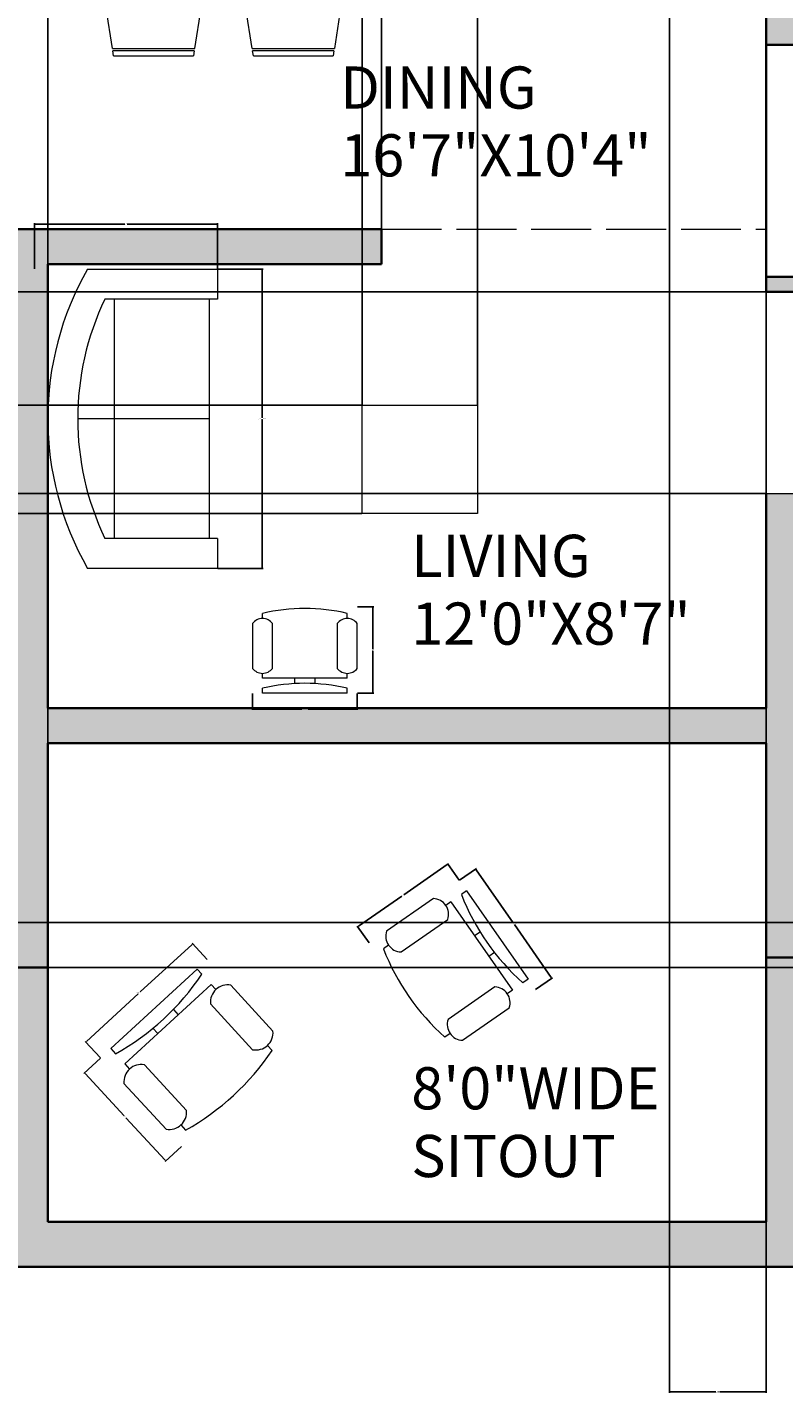
# Model space of a CAD drawing. Units: inches. Extents: x -12 to 539, y -477 to 51.
# Tile 3 of 6: x 173 to 325, y -477 to -203. Entities that reach past the tile are written whole.
import ezdxf

# ---------------------------------------------------------------- set-up
doc = ezdxf.new("R2010")
doc.units = ezdxf.units.IN
doc.header["$MEASUREMENT"] = 0
doc.linetypes.add('ACAD_ISO02W100', pattern=[15, 12, -3])
for name, color, linetype, lineweight in [('A-ANNO-DIMS', 2, 'Continuous', 18), ('A-AREA-IDEN', 7, 'Continuous', 18), ('A-FLOR-CASE', 9, 'Continuous', 18), ('A-FURN', 8, 'Continuous', 18), ('A-WALL', 7, 'Continuous', 35), ('A-WALL-OVHD', 7, 'ACAD_ISO02W100', 18)]:
    doc.layers.add(name, color=color, linetype=linetype, lineweight=lineweight)
doc.layers.add('A-WALL-PATT', color=252, linetype='Continuous', lineweight=13, true_color=0x939598)
doc.styles.get("Standard").update_dxf_attribs({"font": 'arial.ttf'})
doc.dimstyles.get("Standard").update_dxf_attribs({"dimtxt": 0.18, "dimasz": 0.18, "dimexe": 0.18, "dimexo": 0.0625, "dimgap": 0.09, "dimtad": 0, "dimtih": 1, "dimtoh": 1, "dimdec": 0, "dimzin": 0, "dimdsep": 46, "dimlunit": 3, "dimtxsty": 'Standard', "dimcen": 0.09, "dimadec": 0, "dimazin": 0, "dimtfac": 1, "dimtdec": 0, "dimtofl": 0, "dimtmove": 0, "dimatfit": 3, "dimfxl": 1, "dimtolj": 1, "dimtzin": 0, "dimarcsym": 0})

# ---------------------------------------------------------------- blocks, each defined once
blk = doc.blocks.new('Dining Set - 36 x 72 in.')
for p, q in [((-22, 27.5), (-22.1562, 26.50042)), ((-22, 27.5), (-6, 27.5)), ((-5.8437, 26.49966), (-6, 27.5)), ((6, 27.5), (5.8438, 26.50042)), ((6, 27.5), (22, 27.5)), ((22.1563, 26.49966), (22, 27.5)), ((-22.2343, 26.00059), (-23.4847, 17.99762)), ((-22.2304, 26), (-5.7608, 26)), ((-5.8416, 26.5), (-22.1534, 26.5)), ((-4.5152, 17.99762), (-5.7655, 25.99926)), ((5.7657, 26.00059), (4.5153, 17.99762)), ((5.7696, 26), (22.2392, 26)), ((22.1584, 26.5), (5.8466, 26.5)), ((23.4848, 17.99762), (22.2345, 25.99926)), ((36, 18), (-36, 18)), ((-36, 18), (-36, -18)), ((36, -18), (36, 18)), ((-44.0006, 8.23428), (-35.9976, 9.48474)), ((-44, 8.23041), (-44, -8.23915)), ((44.0006, 8.23428), (35.9976, 9.48474)), ((44, 8.23041), (44, -8.23915)), ((-45.5, 8), (-44.5004, 8.15617)), ((-45.5, 8), (-45.5, -8)), ((-44.5, -8.15843), (-44.5, 8.15338)), ((44.5, -8.15843), (44.5, 8.15338)), ((45.5, 8), (44.5005, 8.15617)), ((45.5, 8), (45.5, -8)), ((-44.4997, -8.15631), (-45.5, -8)), ((44.4997, -8.15631), (45.5, -8)), ((-35.9976, -9.48476), (-43.9993, -8.2345)), ((35.9976, -9.48476), (43.9993, -8.2345)), ((-36, -18), (36, -18)), ((-22.2343, -26.0006), (-23.4847, -17.99762)), ((-4.5152, -17.99762), (-5.7655, -25.99928)), ((5.7657, -26.0006), (4.5153, -17.99762)), ((23.4848, -17.99762), (22.2345, -25.99928)), ((-22.2304, -26), (-5.7608, -26)), ((-22, -27.5), (-22.1562, -26.50044)), ((-5.8416, -26.5), (-22.1534, -26.5)), ((-5.8437, -26.49967), (-6, -27.5)), ((5.7696, -26), (22.2392, -26)), ((6, -27.5), (5.8438, -26.50044)), ((22.1584, -26.5), (5.8466, -26.5)), ((22.1563, -26.49967), (22, -27.5)), ((-22, -27.5), (-6, -27.5)), ((6, -27.5), (22, -27.5))]:
    blk.add_line(p, q)
for points in [[(-36, 15), (-31.1772, 14.97754), (-26.8079, 14.91406), (-22.8538, 14.81543), (-19.276, 14.6875), (-16.0362, 14.53613), (-13.0957, 14.36718), (-10.4159, 14.18652), (-7.9583, 14), (-5.6904, 13.81315), (-3.6035, 13.63021), (-1.6954, 13.45508), (0.0365, 13.29166), (1.5945, 13.14388), (2.9811, 13.01562), (4.1988, 12.9108), (5.25, 12.83333), (6.1393, 12.78613), (6.8802, 12.76823), (7.4883, 12.77767), (7.9792, 12.8125), (8.3685, 12.87077), (8.6719, 12.95052), (8.9049, 13.0498), (9.0833, 13.16666), (9.2205, 13.29899), (9.3216, 13.44401), (9.3895, 13.59879), (9.4271, 13.76041), (9.4373, 13.92594), (9.4232, 14.09245), (9.3875, 14.257), (9.3333, 14.41666), (9.2638, 14.56917), (9.1836, 14.71484), (9.0975, 14.85465), (9.0104, 14.98958), (8.9272, 15.1206), (8.8529, 15.2487), (8.7922, 15.37483), (8.75, 15.5), (8.7305, 15.62467), (8.7344, 15.74739), (8.7617, 15.86621), (8.8125, 15.97916), (8.8867, 16.08431), (8.9844, 16.17968), (9.1055, 16.26334), (9.25, 16.33333), (9.4189, 16.38802), (9.6172, 16.42708), (9.8506, 16.45052), (10.125, 16.45833), (10.4463, 16.45052), (10.8203, 16.42708), (11.2529, 16.38802), (11.75, 16.33333), (12.3184, 16.26318), (12.9694, 16.17838), (13.7151, 16.07991), (14.5677, 15.96875), (15.5395, 15.84586), (16.6426, 15.71224), (17.8893, 15.56884), (19.2917, 15.41666), (20.859, 15.25667), (22.5879, 15.08984), (24.4721, 14.91715), (26.5052, 14.73958), (28.6809, 14.5581), (30.9929, 14.3737), (33.4347, 14.18733), (36, 14)], [(-36, 10), (-28.9766, 10.14274), (-23.1725, 10.20442), (-18.4241, 10.19775), (-14.5677, 10.13541), (-11.4399, 10.03011), (-8.877, 9.89453), (-6.7154, 9.74137), (-4.7917, 9.58333), (-2.9698, 9.43082), (-1.2246, 9.28515), (0.4415, 9.14534), (2.026, 9.01041), (3.5266, 8.87939), (4.9408, 8.7513), (6.266, 8.62516), (7.5, 8.5), (8.6411, 8.37549), (9.6914, 8.2539), (10.6538, 8.13818), (11.5312, 8.03125), (12.3267, 7.93603), (13.043, 7.85547), (13.6831, 7.79248), (14.25, 7.75), (14.7471, 7.7303), (15.1797, 7.73307), (15.5537, 7.75732), (15.875, 7.80208), (16.1494, 7.86637), (16.3828, 7.94922), (16.5811, 8.04964), (16.75, 8.16666), (16.8944, 8.29915), (17.0143, 8.44531), (17.1089, 8.60319), (17.1771, 8.77083), (17.218, 8.94629), (17.2305, 9.1276), (17.2137, 9.31282), (17.1667, 9.5), (17.0895, 9.6875), (16.987, 9.875), (16.8649, 10.0625), (16.7292, 10.25), (16.5856, 10.4375), (16.4401, 10.625), (16.2985, 10.8125), (16.1667, 11), (16.05, 11.18733), (15.9518, 11.3737), (15.8752, 11.5581), (15.8229, 11.73958), (15.798, 11.91715), (15.8034, 12.08984), (15.842, 12.25667), (15.9167, 12.41666), (16.0295, 12.56836), (16.1784, 12.70833), (16.3605, 12.83268), (16.5729, 12.9375), (16.8127, 13.01888), (17.0768, 13.07291), (17.3625, 13.0957), (17.6667, 13.08333), (17.9894, 13.03312), (18.3418, 12.94726), (18.7382, 12.82918), (19.1927, 12.68229), (19.7195, 12.51001), (20.3327, 12.31575), (21.0465, 12.10294), (21.875, 11.875), (22.8357, 11.63354), (23.959, 11.37304), (25.2786, 11.08618), (26.8282, 10.76562), (28.6414, 10.40405), (30.752, 9.99414), (33.1936, 9.52856), (36, 9)], [(-36, 5.5), (-30.7157, 5.3348), (-26.069, 5.20963), (-21.9946, 5.11767), (-18.4271, 5.05208), (-15.3009, 5.00602), (-12.5508, 4.97265), (-10.1112, 4.94515), (-7.9167, 4.91666), (-5.909, 4.88167), (-4.0586, 4.83984), (-2.3429, 4.79215), (-0.7396, 4.73958), (0.7739, 4.6831), (2.22, 4.6237), (3.6213, 4.56233), (5, 4.5), (6.373, 4.43782), (7.7344, 4.3776), (9.0723, 4.32129), (10.375, 4.27083), (11.6309, 4.22819), (12.8281, 4.19531), (13.9551, 4.17415), (15, 4.16666), (15.954, 4.17448), (16.819, 4.19791), (17.6001, 4.23698), (18.3021, 4.29166), (18.9299, 4.36198), (19.4883, 4.44791), (19.9823, 4.54948), (20.4167, 4.66666), (20.7969, 4.79899), (21.1302, 4.94401), (21.4245, 5.09879), (21.6875, 5.26041), (21.9271, 5.42594), (22.1511, 5.59245), (22.3672, 5.757), (22.5834, 5.91666), (22.8065, 6.06868), (23.0404, 6.21093), (23.2879, 6.34147), (23.5521, 6.45833), (23.8358, 6.55957), (24.142, 6.64323), (24.4735, 6.70735), (24.8334, 6.75), (25.2235, 6.76969), (25.642, 6.76692), (26.0858, 6.74267), (26.5521, 6.69791), (27.0379, 6.63362), (27.5404, 6.55078), (28.0565, 6.45036), (28.5834, 6.33333), (29.1242, 6.19987), (29.7071, 6.04687), (30.3661, 5.87044), (31.1354, 5.66666), (32.0493, 5.43164), (33.142, 5.16146), (34.4475, 4.85221), (36, 4.5)], [(-36, -1), (-30.7915, -0.6591), (-26.0195, -0.38216), (-21.6519, -0.16284), (-17.6563, 0.00521), (-14.0005, 0.12833), (-10.6523, 0.21289), (-7.5796, 0.26522), (-4.75, 0.29166), (-2.134, 0.29793), (0.2878, 0.28711), (2.5317, 0.26163), (4.6146, 0.22396), (6.5529, 0.17651), (8.3633, 0.12174), (10.0623, 0.06209), (11.6667, 0), (13.1899, -0.06201), (14.6341, -0.1211), (15.9982, -0.17432), (17.2813, -0.21875), (18.4823, -0.25147), (19.6003, -0.26953), (20.6343, -0.27002), (21.5834, -0.25), (22.4481, -0.20768), (23.2357, -0.14584), (23.9549, -0.06836), (24.6146, 0.02083), (25.2235, 0.11784), (25.7904, 0.21875), (26.3241, 0.31966), (26.8334, 0.41666), (27.3265, 0.50618), (27.8099, 0.58593), (28.2894, 0.65397), (28.7709, 0.70833), (29.2601, 0.74707), (29.763, 0.76823), (30.2855, 0.76985), (30.8334, 0.75), (31.4088, 0.70784), (31.9994, 0.64713), (32.589, 0.57275), (33.1615, 0.48958), (33.7008, 0.4025), (34.1908, 0.3164), (34.6153, 0.23616), (34.9584, 0.16666), (35.2099, 0.11165), (35.3848, 0.07031), (35.504, 0.04069), (35.5886, 0.02083), (35.6594, 0.00879), (35.7377, 0.0026), (35.8442, 0.00032), (36, 0)], [(-36, -6.5), (-27.1843, -6.31267), (-20.084, -6.1263), (-14.469, -5.9419), (-10.1094, -5.76042), (-6.7752, -5.58285), (-4.2363, -5.41016), (-2.2629, -5.24333), (-0.625, -5.08334), (0.8708, -4.93099), (2.2715, -4.78646), (3.5872, -4.64974), (4.8281, -4.52084), (6.0046, -4.39974), (7.127, -4.28646), (8.2053, -4.18099), (9.25, -4.08334), (10.2705, -3.99382), (11.2734, -3.91407), (12.2647, -3.84603), (13.25, -3.79167), (14.2354, -3.75293), (15.2266, -3.73177), (16.2295, -3.73015), (17.25, -3.75), (18.2912, -3.79248), (19.3451, -3.85547), (20.4009, -3.93604), (21.4479, -4.03125), (22.4754, -4.13819), (23.4727, -4.25391), (24.4289, -4.37549), (25.3334, -4.5), (26.1785, -4.62492), (26.9694, -4.74935), (27.7145, -4.87281), (28.4219, -4.99479), (29.1, -5.11483), (29.7572, -5.23242), (30.4016, -5.34709), (31.0417, -5.45834), (31.6837, -5.56437), (32.3262, -5.65821), (32.9658, -5.73153), (33.599, -5.77604), (34.2224, -5.78345), (34.8327, -5.74545), (35.4264, -5.65373), (36, -5.5)], [(-36, -10), (-26.4022, -9.81299), (-18.4675, -9.62891), (-11.9839, -9.45069), (-6.7396, -9.28125), (-2.5226, -9.12354), (0.8789, -8.98047), (3.6769, -8.85498), (6.0833, -8.75), (8.2767, -8.66765), (10.3021, -8.60677), (12.1712, -8.56543), (13.8958, -8.54167), (15.4876, -8.53353), (16.9583, -8.53907), (18.3197, -8.55632), (19.5834, -8.58334), (20.7616, -8.61841), (21.8685, -8.66081), (22.9188, -8.71004), (23.9271, -8.76563), (24.9081, -8.82707), (25.8763, -8.89388), (26.8465, -8.96558), (27.8334, -9.04167), (28.8474, -9.12118), (29.8828, -9.20117), (30.93, -9.27824), (31.9792, -9.34896), (33.0205, -9.40991), (34.0443, -9.45768), (35.0407, -9.48885), (36, -9.5)], [(-36, -14.5), (-30.0881, -14.33513), (-25.0332, -14.21224), (-20.7312, -14.12647), (-17.0781, -14.07292), (-13.97, -14.04671), (-11.3027, -14.04297), (-8.9724, -14.05681), (-6.875, -14.08334), (-4.9224, -14.11833), (-3.0905, -14.16016), (-1.3709, -14.20785), (0.2448, -14.26042), (1.7647, -14.3169), (3.1973, -14.3763), (4.5507, -14.43767), (5.8333, -14.5), (7.0554, -14.5621), (8.235, -14.62175), (9.3922, -14.67652), (10.5469, -14.72396), (11.7192, -14.76164), (12.929, -14.78711), (14.1965, -14.79794), (15.5417, -14.79167), (16.9933, -14.76424), (18.6152, -14.70508), (20.4804, -14.60197), (22.6615, -14.44271), (25.2312, -14.21509), (28.2624, -13.9069), (31.8277, -13.50594), (36, -13)]]:
    blk.add_lwpolyline(points)
blk = doc.blocks.new('Sofa - Roundback Loveseat 5 ft.')
for p, q in [((0, -32.44198), (0, -5.99998)), ((-24, -33.99998), (-24, -11.46958)), ((-23.9998, -13.38178), (23.99986, -13.38178)), ((24.00004, -33.99998), (24.00004, -11.46958)), ((-24, -32.44198), (24.00004, -32.44198))]:
    blk.add_line(p, q)
for points in [[(-24, -33.99998), (-30, -33.99998), (-30, -7.99998)], [(30.00004, -7.99998), (30.00004, -33.99998), (24.00004, -33.99998)]]:
    blk.add_lwpolyline(points)
for centre, radius, start, end in [((0, -60.24998), 60.24998, 60.13715, 119.8628), ((0, -61.38438), 55.38444, 64.32083, 115.6792)]:
    blk.add_arc(centre, radius, start, end)
blk = doc.blocks.new('Chair - Desk')
for p, q in [((-8.5, 0), (-8.5, -1)), ((-8.5, 0), (8.5, 0)), ((8.5, 0), (8.5, -1)), ((-2, -3), (-2, -1.9355)), ((2, -1.9576), (2, -3)), ((-8.5, -3), (-8.5, -4)), ((-8.5, -3), (8.5, -3)), ((8.5, -3), (8.5, -4)), ((-10.5, -5), (-10.5, -14)), ((-6.5, -14), (-6.5, -5)), ((6.5, -5), (6.5, -14)), ((10.5, -14), (10.5, -5)), ((-8.5, -15), (-8.5, -16)), ((8.5, -15), (8.5, -16))]:
    blk.add_line(p, q)
for centre, radius, start, end in [((0, 34.625), 36.625, 256.5803, 283.4197), ((-8.5, -6.5), 2.5, 36.8699, 143.1301), ((8.5, -6.5), 2.5, 36.8699, 143.1301), ((-8.5, -12.5), 2.5, 216.8699, 323.1301), ((8.5, -12.5), 2.5, 216.8699, 323.1301), ((0, 19.625), 36.625, 256.5803, 283.4197)]:
    blk.add_arc(centre, radius, start, end)
blk = doc.blocks.new('*D13')
at = {"layer": 'A-ANNO-DIMS', "color": 0, "lineweight": -2, "transparency": 16777216}
for p, q in [((218.14, -337.07), (218.14, -340.34)), ((239.14, -337.07), (239.14, -340.34)), ((218.32, -340.16), (228.02, -340.16)), ((238.96, -340.16), (229.27, -340.16))]:
    blk.add_line(p, q, dxfattribs=at)
at = {"layer": 'A-ANNO-DIMS', "color": 0, "transparency": 16777216}
for points in [[(218.32, -340.13), (218.32, -340.19), (218.14, -340.16)], [(238.96, -340.13), (238.96, -340.19), (239.14, -340.16)]]:
    blk.add_solid(points, dxfattribs=at)
at = {"layer": 'Defpoints', "color": 0, "transparency": 16777216}
for p in [(218.14, -337.01), (239.14, -337.01), (218.14, -340.16)]:
    blk.add_point(p, dxfattribs=at)
at = {"layer": 'A-ANNO-DIMS', "color": 0, "transparency": 16777216, "insert": (228.64, -340.16), "char_height": 0.18, "attachment_point": 5}
blk.add_mtext('\\A1;CHAIR 21', dxfattribs=at)
blk = doc.blocks.new('*D14')
at = {"layer": 'A-ANNO-DIMS', "color": 0, "lineweight": -2, "transparency": 16777216}
for p, q in [((239.21, -319.67), (242.47, -319.67)), ((242.29, -319.85), (242.29, -328.16)), ((242.29, -336.83), (242.29, -328.52)), ((239.21, -337.01), (242.47, -337.01))]:
    blk.add_line(p, q, dxfattribs=at)
at = {"layer": 'A-ANNO-DIMS', "color": 0, "transparency": 16777216}
for points in [[(242.26, -319.85), (242.32, -319.85), (242.29, -319.67)], [(242.26, -336.83), (242.32, -336.83), (242.29, -337.01)]]:
    blk.add_solid(points, dxfattribs=at)
at = {"layer": 'Defpoints', "color": 0, "transparency": 16777216}
for p in [(239.14, -319.67), (239.14, -337.01), (242.29, -337.01)]:
    blk.add_point(p, dxfattribs=at)
at = {"layer": 'A-ANNO-DIMS', "color": 0, "transparency": 16777216, "insert": (242.29, -328.34), "char_height": 0.18, "attachment_point": 5}
blk.add_mtext('\\A1;17', dxfattribs=at)
blk = doc.blocks.new('*D15')
at = {"layer": 'A-ANNO-DIMS', "color": 0, "lineweight": -2, "transparency": 16777216}
for p, q in [((206.03, -387.34), (195.65, -396.89)), ((209.07, -390.39), (206.04, -387.09)), ((184.87, -406.8), (195.25, -397.25)), ((187.65, -410.08), (184.62, -406.79))]:
    blk.add_line(p, q, dxfattribs=at)
at = {"layer": 'A-ANNO-DIMS', "color": 0, "transparency": 16777216}
for points in [[(206.01, -387.32), (206.05, -387.37), (206.16, -387.22)], [(184.85, -406.77), (184.9, -406.82), (184.74, -406.92)]]:
    blk.add_solid(points, dxfattribs=at)
at = {"layer": 'Defpoints', "color": 0, "transparency": 16777216}
for p in [(206.16, -387.22), (209.11, -390.44), (187.7, -410.13)]:
    blk.add_point(p, dxfattribs=at)
at = {"layer": 'A-ANNO-DIMS', "color": 0, "transparency": 16777216, "insert": (195.45, -397.07), "char_height": 0.18, "attachment_point": 5}
blk.add_mtext('\\A1;CHAIR 29', dxfattribs=at)
blk = doc.blocks.new('*D16')
at = {"layer": 'A-ANNO-DIMS', "color": 0, "lineweight": -2, "transparency": 16777216}
for p, q in [((187.65, -410.17), (184.35, -413.21)), ((184.61, -413.22), (192.45, -421.74)), ((200.62, -430.63), (192.78, -422.1)), ((203.91, -427.85), (200.61, -430.88))]:
    blk.add_line(p, q, dxfattribs=at)
at = {"layer": 'A-ANNO-DIMS', "color": 0, "transparency": 16777216}
for points in [[(184.63, -413.2), (184.58, -413.24), (184.48, -413.08)], [(200.64, -430.61), (200.6, -430.65), (200.74, -430.76)]]:
    blk.add_solid(points, dxfattribs=at)
at = {"layer": 'Defpoints', "color": 0, "transparency": 16777216}
for p in [(187.7, -410.13), (184.48, -413.08), (203.95, -427.81)]:
    blk.add_point(p, dxfattribs=at)
at = {"layer": 'A-ANNO-DIMS', "color": 0, "transparency": 16777216, "insert": (192.61, -421.92), "char_height": 0.18, "attachment_point": 5}
blk.add_mtext('\\A1;24', dxfattribs=at)
blk = doc.blocks.new('*D17')
at = {"layer": 'A-ANNO-DIMS', "color": 0, "lineweight": -2, "transparency": 16777216}
for p, q in [((259.65, -374.5), (263.03, -372.15)), ((262.99, -372.4), (270.37, -383.02)), ((278.01, -394), (270.62, -383.38)), ((274.88, -396.39), (278.26, -394.04))]:
    blk.add_line(p, q, dxfattribs=at)
at = {"layer": 'A-ANNO-DIMS', "color": 0, "transparency": 16777216}
for points in [[(263.01, -372.39), (262.96, -372.42), (262.88, -372.26)], [(278.03, -393.98), (277.98, -394.01), (278.11, -394.14)]]:
    blk.add_solid(points, dxfattribs=at)
at = {"layer": 'Defpoints', "color": 0, "transparency": 16777216}
for p in [(259.6, -374.54), (278.11, -394.14), (274.83, -396.43)]:
    blk.add_point(p, dxfattribs=at)
at = {"layer": 'A-ANNO-DIMS', "color": 0, "transparency": 16777216, "insert": (270.5, -383.2), "char_height": 0.18, "attachment_point": 5}
blk.add_mtext('\\A1;CHAIR 27', dxfattribs=at)
blk = doc.blocks.new('*D18')
at = {"layer": 'A-ANNO-DIMS', "color": 0, "lineweight": -2, "transparency": 16777216}
for p, q in [((257.17, -371.36), (248.5, -377.39)), ((259.56, -374.49), (257.21, -371.11)), ((239.4, -383.72), (248.06, -377.69)), ((241.5, -387.06), (239.15, -383.68))]:
    blk.add_line(p, q, dxfattribs=at)
at = {"layer": 'A-ANNO-DIMS', "color": 0, "transparency": 16777216}
for points in [[(257.15, -371.34), (257.18, -371.38), (257.32, -371.26)], [(239.38, -383.7), (239.41, -383.75), (239.25, -383.83)]]:
    blk.add_solid(points, dxfattribs=at)
at = {"layer": 'Defpoints', "color": 0, "transparency": 16777216}
for p in [(257.32, -371.26), (259.6, -374.54), (241.53, -387.11)]:
    blk.add_point(p, dxfattribs=at)
at = {"layer": 'A-ANNO-DIMS', "color": 0, "transparency": 16777216, "insert": (248.28, -377.54), "char_height": 0.18, "attachment_point": 5}
blk.add_mtext('\\A1;22', dxfattribs=at)
blk = doc.blocks.new('*D33')
at = {"layer": 'A-ANNO-DIMS', "color": 0, "lineweight": -2, "transparency": 16777216}
for p, q in [((211.17, -251.96), (220.28, -251.96)), ((220.1, -252.14), (220.1, -281.78)), ((220.1, -311.78), (220.1, -282.14)), ((211.17, -311.96), (220.28, -311.96))]:
    blk.add_line(p, q, dxfattribs=at)
at = {"layer": 'A-ANNO-DIMS', "color": 0, "transparency": 16777216}
for points in [[(220.07, -252.14), (220.13, -252.14), (220.1, -251.96)], [(220.07, -311.78), (220.13, -311.78), (220.1, -311.96)]]:
    blk.add_solid(points, dxfattribs=at)
at = {"layer": 'Defpoints', "color": 0, "transparency": 16777216}
for p in [(211.1, -251.96), (220.1, -251.96), (211.1, -311.96)]:
    blk.add_point(p, dxfattribs=at)
at = {"layer": 'A-ANNO-DIMS', "color": 0, "transparency": 16777216, "insert": (220.1, -281.96), "char_height": 0.18, "attachment_point": 5}
blk.add_mtext('\\A1;LOVESEAT 60', dxfattribs=at)
blk = doc.blocks.new('*D34')
at = {"layer": 'A-ANNO-DIMS', "color": 0, "lineweight": -2, "transparency": 16777216}
for p, q in [((174.44, -251.9), (174.44, -242.78)), ((174.62, -242.96), (192.55, -242.96)), ((210.92, -242.96), (192.99, -242.96)), ((211.1, -251.9), (211.1, -242.78))]:
    blk.add_line(p, q, dxfattribs=at)
at = {"layer": 'A-ANNO-DIMS', "color": 0, "transparency": 16777216}
for points in [[(174.62, -242.93), (174.62, -242.99), (174.44, -242.96)], [(210.92, -242.93), (210.92, -242.99), (211.1, -242.96)]]:
    blk.add_solid(points, dxfattribs=at)
at = {"layer": 'Defpoints', "color": 0, "transparency": 16777216}
for p in [(174.44, -242.96), (174.44, -251.96), (211.1, -251.96)]:
    blk.add_point(p, dxfattribs=at)
at = {"layer": 'A-ANNO-DIMS', "color": 0, "transparency": 16777216, "insert": (192.77, -242.96), "char_height": 0.18, "attachment_point": 5}
blk.add_mtext('\\A1;37', dxfattribs=at)
blk = doc.blocks.new('*D35')
at = {"layer": 'A-ANNO-DIMS', "color": 0, "lineweight": -2, "transparency": 16777216}
for p, q in [((301.71, 16.95), (301.71, -477.23)), ((321.1, 16.95), (321.1, -477.23)), ((301.89, -477.05), (311.02, -477.05)), ((320.92, -477.05), (311.79, -477.05))]:
    blk.add_line(p, q, dxfattribs=at)
at = {"layer": 'A-ANNO-DIMS', "color": 0, "transparency": 16777216}
for points in [[(301.89, -477.02), (301.89, -477.08), (301.71, -477.05)], [(320.92, -477.02), (320.92, -477.08), (321.1, -477.05)]]:
    blk.add_solid(points, dxfattribs=at)
at = {"layer": 'Defpoints', "color": 0, "transparency": 16777216}
for p in [(301.71, 17.01), (321.1, 17.01), (321.1, -477.05)]:
    blk.add_point(p, dxfattribs=at)
at = {"layer": 'A-ANNO-DIMS', "color": 0, "transparency": 16777216, "insert": (311.41, -477.05), "char_height": 0.18, "attachment_point": 5}
blk.add_mtext('\\A1;19.39', dxfattribs=at)
blk = doc.blocks.new('*D42')
at = {"layer": 'A-ANNO-DIMS', "color": 0, "lineweight": -2, "transparency": 16777216}
for p, q in [((177.1, -442.93), (177.1, 51.25)), ((177.28, 51.07), (248.82, 51.07)), ((320.92, 51.07), (249.38, 51.07)), ((321.1, -442.93), (321.1, 51.25))]:
    blk.add_line(p, q, dxfattribs=at)
at = {"layer": 'A-ANNO-DIMS', "color": 0, "transparency": 16777216}
for points in [[(177.28, 51.1), (177.28, 51.04), (177.1, 51.07)], [(320.92, 51.1), (320.92, 51.04), (321.1, 51.07)]]:
    blk.add_solid(points, dxfattribs=at)
at = {"layer": 'Defpoints', "color": 0, "transparency": 16777216}
for p in [(321.1, 51.07), (177.1, -442.99), (321.1, -442.99)]:
    blk.add_point(p, dxfattribs=at)
at = {"layer": 'A-ANNO-DIMS', "color": 0, "transparency": 16777216, "insert": (249.1, 51.07), "char_height": 0.18, "attachment_point": 5}
blk.add_mtext('\\A1;144', dxfattribs=at)
blk = doc.blocks.new('*D45')
at = {"layer": 'A-ANNO-DIMS', "color": 0, "lineweight": -2, "transparency": 16777216}
for p, q in [((22.17, -382.99), (539.23, -382.99)), ((539.05, -383.17), (539.05, -387.31)), ((539.05, -391.81), (539.05, -387.67)), ((13.17, -391.99), (539.23, -391.99))]:
    blk.add_line(p, q, dxfattribs=at)
at = {"layer": 'A-ANNO-DIMS', "color": 0, "transparency": 16777216}
for points in [[(539.02, -383.17), (539.08, -383.17), (539.05, -382.99)], [(539.02, -391.81), (539.08, -391.81), (539.05, -391.99)]]:
    blk.add_solid(points, dxfattribs=at)
at = {"layer": 'Defpoints', "color": 0, "transparency": 16777216}
for p in [(22.1, -382.99), (539.05, -382.99), (13.1, -391.99)]:
    blk.add_point(p, dxfattribs=at)
at = {"layer": 'A-ANNO-DIMS', "color": 0, "transparency": 16777216, "insert": (539.05, -387.49), "char_height": 0.18, "attachment_point": 5}
blk.add_mtext('\\A1;9', dxfattribs=at)
blk = doc.blocks.new('*D54')
at = {"layer": 'A-ANNO-DIMS', "color": 0, "lineweight": -2, "transparency": 16777216}
for p, q in [((321.04, -256.55), (-12.14, -256.55)), ((-11.96, -256.73), (-11.96, -276.57)), ((-11.96, -296.78), (-11.96, -276.93)), ((321.04, -296.96), (-12.14, -296.96))]:
    blk.add_line(p, q, dxfattribs=at)
at = {"layer": 'A-ANNO-DIMS', "color": 0, "transparency": 16777216}
for points in [[(-11.99, -256.73), (-11.93, -256.73), (-11.96, -256.55)], [(-11.99, -296.78), (-11.93, -296.78), (-11.96, -296.96)]]:
    blk.add_solid(points, dxfattribs=at)
at = {"layer": 'Defpoints', "color": 0, "transparency": 16777216}
for p in [(321.1, -256.55), (-11.96, -296.96), (321.1, -296.96)]:
    blk.add_point(p, dxfattribs=at)
at = {"layer": 'A-ANNO-DIMS', "color": 0, "transparency": 16777216, "insert": (-11.96, -276.75), "char_height": 0.18, "attachment_point": 5}
blk.add_mtext('\\A1;40.41', dxfattribs=at)
blk = doc.blocks.new('*D56')
at = {"layer": 'A-ANNO-DIMS', "color": 0, "lineweight": -2, "transparency": 16777216}
for p, q in [((321.1, -256.48), (321.1, 51.25)), ((321.28, 51.07), (336.1, 51.07)), ((351.7, 51.07), (336.89, 51.07)), ((351.88, -256.48), (351.88, 51.25))]:
    blk.add_line(p, q, dxfattribs=at)
at = {"layer": 'A-ANNO-DIMS', "color": 0, "transparency": 16777216}
for points in [[(321.28, 51.1), (321.28, 51.04), (321.1, 51.07)], [(351.7, 51.1), (351.7, 51.04), (351.88, 51.07)]]:
    blk.add_solid(points, dxfattribs=at)
at = {"layer": 'Defpoints', "color": 0, "transparency": 16777216}
for p in [(351.88, 51.07), (321.1, -256.55), (351.88, -256.55)]:
    blk.add_point(p, dxfattribs=at)
at = {"layer": 'A-ANNO-DIMS', "color": 0, "transparency": 16777216, "insert": (336.49, 51.07), "char_height": 0.18, "attachment_point": 5}
blk.add_mtext('\\A1;30.78', dxfattribs=at)
blk = doc.blocks.new('*D58')
at = {"layer": 'A-ANNO-DIMS', "color": 0, "lineweight": -2, "transparency": 16777216}
for p, q in [((177.1, -250.93), (177.1, 51.25)), ((177.28, 51.07), (210.17, 51.07)), ((243.85, 51.07), (210.96, 51.07)), ((244.03, -250.93), (244.03, 51.25))]:
    blk.add_line(p, q, dxfattribs=at)
at = {"layer": 'A-ANNO-DIMS', "color": 0, "transparency": 16777216}
for points in [[(177.28, 51.1), (177.28, 51.04), (177.1, 51.07)], [(243.85, 51.1), (243.85, 51.04), (244.03, 51.07)]]:
    blk.add_solid(points, dxfattribs=at)
at = {"layer": 'Defpoints', "color": 0, "transparency": 16777216}
for p in [(244.03, 51.07), (177.1, -250.99), (244.03, -250.99)]:
    blk.add_point(p, dxfattribs=at)
at = {"layer": 'A-ANNO-DIMS', "color": 0, "transparency": 16777216, "insert": (210.56, 51.07), "char_height": 0.18, "attachment_point": 5}
blk.add_mtext('\\A1;66.92', dxfattribs=at)
blk = doc.blocks.new('*D59')
at = {"layer": 'A-ANNO-DIMS', "color": 0, "lineweight": -2, "transparency": 16777216}
for p, q in [((240.14, -279.15), (240.14, 51.25)), ((240.32, 51.07), (251.3, 51.07)), ((263.07, 51.07), (252.09, 51.07)), ((263.25, -279.15), (263.25, 51.25))]:
    blk.add_line(p, q, dxfattribs=at)
at = {"layer": 'A-ANNO-DIMS', "color": 0, "transparency": 16777216}
for points in [[(240.32, 51.1), (240.32, 51.04), (240.14, 51.07)], [(263.07, 51.1), (263.07, 51.04), (263.25, 51.07)]]:
    blk.add_solid(points, dxfattribs=at)
at = {"layer": 'Defpoints', "color": 0, "transparency": 16777216}
for p in [(263.25, 51.07), (240.14, -279.21), (263.25, -279.21)]:
    blk.add_point(p, dxfattribs=at)
at = {"layer": 'A-ANNO-DIMS', "color": 0, "transparency": 16777216, "insert": (251.69, 51.07), "char_height": 0.18, "attachment_point": 5}
blk.add_mtext('\\A1;23.12', dxfattribs=at)
blk = doc.blocks.new('*D60')
at = {"layer": 'A-ANNO-DIMS', "color": 0, "lineweight": -2, "transparency": 16777216}
for p, q in [((240.07, -279.21), (-12.14, -279.21)), ((-11.96, -279.39), (-11.96, -289.91)), ((-11.96, -300.79), (-11.96, -290.27)), ((240.07, -300.97), (-12.14, -300.97))]:
    blk.add_line(p, q, dxfattribs=at)
at = {"layer": 'A-ANNO-DIMS', "color": 0, "transparency": 16777216}
for points in [[(-11.99, -279.39), (-11.93, -279.39), (-11.96, -279.21)], [(-11.99, -300.79), (-11.93, -300.79), (-11.96, -300.97)]]:
    blk.add_solid(points, dxfattribs=at)
at = {"layer": 'Defpoints', "color": 0, "transparency": 16777216}
for p in [(240.14, -279.21), (-11.96, -300.97), (240.14, -300.97)]:
    blk.add_point(p, dxfattribs=at)
at = {"layer": 'A-ANNO-DIMS', "color": 0, "transparency": 16777216, "insert": (-11.96, -290.09), "char_height": 0.18, "attachment_point": 5}
blk.add_mtext('\\A1;21.76', dxfattribs=at)

msp = doc.modelspace()

# ---------------------------------------------------------------- hatches: boundary and pattern name
at = {"layer": 'A-WALL-PATT'}
h = msp.add_hatch(color=256, dxfattribs=at)
h.dxf.hatch_style = 1
h.paths.add_polyline_path([(267.143, 26.0124), (13.1031, 26.0124), (13.1031, -391.9876), (177.1031, -391.9876), (177.1031, -346.9876), (307.7315, -346.9876), (321.1031, -346.9876), (321.1031, -389.9876), (469.1031, -389.9876), (469.1031, 26.0124), (302.7142, 26.0124), (302.7142, 17.0124), (321.1031, 17.0124), (321.1031, -131.577, -0.04877504), (328.1031, -132.2621), (328.1031, 17.0124), (460.1031, 17.0124), (460.1031, -124.9876), (382.1031, -124.9876), (379.1031, -124.9876), (379.1031, -131.5624), (382.1031, -131.5624), (382.1031, -127.9876), (460.1031, -127.9876), (460.1031, -153.7747), (460.1031, -199.9876), (382.1031, -199.9876), (382.1031, -167.7132), (379.1031, -167.7132), (379.1031, -199.9876), (328.1031, -199.9876), (328.1031, -167.7132), (321.1031, -167.7132), (321.1031, -206.9876), (460.1031, -206.9876), (460.1031, -323.9876), (388.677, -323.9876, -0.02504709), (388.5266, -326.9876), (460.1031, -326.9876), (460.1031, -380.9876), (328.1031, -380.9876), (328.1031, -326.9876), (358.677, -326.9876), (358.677, -323.9876), (328.1031, -323.9876), (328.1031, -296.9562), (321.1031, -296.9562), (321.1031, -339.9876), (307.7315, -339.9876), (177.1031, -339.9876), (177.1031, -250.9876), (244.0259, -250.9876), (244.0259, -243.9876), (163.7315, -243.9876), (163.7315, -250.9876), (170.1031, -250.9876), (170.1031, -382.9876), (22.1031, -382.9876), (22.1031, -250.9876), (41.3871, -250.9876, -0.06888376), (40.8612, -243.9876), (22.1031, -243.9876), (22.1031, -183.9876), (118.1031, -183.9876), (118.1031, -243.9876), (71.6031, -243.9876), (71.6031, -250.9876), (128.4772, -250.9876, -0.04900189), (127.7315, -243.9876), (121.1031, -243.9876), (121.1031, -183.9876), (121.1031, -120.9876), (118.1031, -120.9876), (118.1031, -180.9876), (22.1031, -180.9876), (22.1031, -120.9876), (49.0045, -120.9876, -0.07000725), (46.9084, -111.9876), (46.1728, -111.9876), (22.1031, -111.9876), (22.1031, 17.0124), (170.1031, 17.0124), (170.1031, -120.9876), (177.1031, -120.9876), (177.1031, 17.0124), (268.2584, 17.0124, -0.0639977)])
h.paths.add_polyline_path([(513.9866, -124.9876), (469.1031, -124.9876), (469.1031, -127.9876), (510.9866, -127.9876), (510.9866, -259.2045), (469.1031, -259.2045), (469.1031, -262.2045), (513.9866, -262.2045)])
h.paths.add_polyline_path([(351.8833, -206.9876), (348.8833, -206.9876), (348.8833, -253.547), (328.1031, -253.547), (321.1031, -253.547), (321.1031, -256.547), (328.1031, -256.547), (351.8833, -256.547)], flags=17)
h.paths.add_polyline_path([(330.1031, -389.9876), (321.1031, -389.9876), (321.1031, -442.9876), (177.1031, -442.9876), (177.1031, -391.9876), (168.1031, -391.9876), (168.1031, -451.9876), (330.1031, -451.9876)])
h.paths.add_polyline_path([(414.1504, -177.6962), (465.5248, -177.6962), (465.5248, -164.7437), (414.1504, -164.7437)], flags=25)

# ---------------------------------------------------------------- linework, layer by layer
at = {"layer": 'A-FLOR-CASE'}
msp.add_line((321.1031, -296.9562), (355.8953, -296.9562), dxfattribs=at)
at = {"layer": 'A-FURN'}
msp.add_lwpolyline([(240.1351, -279.2095), (263.2543, -279.2095), (263.2543, -300.9695), (240.1351, -300.9695)], close=True, dxfattribs=at)
at = {"layer": 'A-WALL'}
for p, q in [((321.1031, -206.9876), (321.1031, -167.7132)), ((460.1031, -206.9876), (321.1031, -206.9876)), ((321.1031, -256.547), (321.1031, -206.9876)), ((163.7315, -243.9876), (244.0259, -243.9876)), ((244.0259, -250.9876), (244.0259, -243.9876)), ((177.1031, -339.9876), (177.1031, -250.9876)), ((177.1031, -250.9876), (244.0259, -250.9876)), ((321.1031, -253.547), (328.1031, -253.547)), ((321.1031, -256.547), (328.1031, -256.547)), ((321.1031, -339.9876), (321.1031, -296.9562)), ((321.1031, -339.9876), (321.1031, -326.9876)), ((307.7315, -339.9876), (177.1031, -339.9876)), ((307.7315, -339.9876), (321.1031, -339.9876)), ((307.7315, -346.9876), (177.1031, -346.9876)), ((177.1031, -391.9876), (177.1031, -346.9876)), ((307.7315, -346.9876), (321.1031, -346.9876)), ((321.1031, -389.9876), (321.1031, -346.9876)), ((321.1031, -346.9876), (321.1031, -442.9876)), ((469.1031, -389.9876), (321.1031, -389.9876)), ((321.1031, -389.9876), (321.1031, -442.9876)), ((13.1031, -391.9876), (177.1031, -391.9876)), ((177.1031, -442.9876), (177.1031, -391.9876)), ((321.1031, -442.9876), (177.1031, -442.9876)), ((330.1031, -451.9876), (168.1031, -451.9876))]:
    msp.add_line(p, q, dxfattribs=at)
at = {"layer": 'A-WALL-OVHD'}
for p, q in [((244.0259, -243.9876), (321.1031, -243.9876)), ((321.1031, -243.9876), (321.1031, -296.9562))]:
    msp.add_line(p, q, dxfattribs=at)

# ---------------------------------------------------------------- block references
at = {"layer": 'A-FURN'}
msp.add_blockref('Dining Set - 36 x 72 in.', (212.314, -181.7338), dxfattribs=at)
for name, p, rotation in [('Sofa - Roundback Loveseat 5 ft.', (177.1031, -281.9586), 90), ('Chair - Desk', (228.6448, -337.0066), 180)]:
    msp.add_blockref(name, p, dxfattribs=dict(at, rotation=rotation))
for p, xscale, yscale, zscale, rotation in [((267.2133, -385.4844), 1.269738823821673, 1.269738823821673, 1.269738823821673, 304.8271913326521), ((198.4054, -400.2831), 1.385542587767751, 1.385542587767751, 1.385542587767751, 42.60131503161123)]:
    msp.add_blockref('Chair - Desk', p, dxfattribs=dict(at, xscale=xscale, yscale=yscale, zscale=zscale, rotation=rotation))

# ---------------------------------------------------------------- texts
at = {"layer": 'A-AREA-IDEN'}
for s, height, p in [('DINING ', 8.45618, (235.7416, -219.7965)), ('16\'7"X10\'4"', 8.456178, (235.7416, -233.3806)), ('LIVING ', 8.45618, (249.9741, -313.6817)), ('12\'0"X8\'7"', 8.45618, (249.9741, -327.2658)), ('8\'0"WIDE', 8.45618, (249.9741, -420.4222)), ('SITOUT', 8.45618, (249.9741, -434.0063))]:
    msp.add_text(s, height=height, dxfattribs=at).set_placement(p)

# ---------------------------------------------------------------- dimensions: what is measured, and where the dimension line sits
at = {"layer": 'A-ANNO-DIMS'}
for base, p1, p2, override, picture, middle in [((321.1031, 51.0724), (177.1031, -442.9876), (321.1031, -442.9876), {"dimdec": 0, "dimlfac": 1, "dimrnd": 0, "dimzin": 0, "dimdsep": 46, "dimlunit": 2}, '*D42', (249.1031, 51.0724)), ((244.0259, 51.0724), (177.1031, -250.9876), (244.0259, -250.9876), {"dimdec": 2, "dimlfac": 1, "dimrnd": 0, "dimzin": 0, "dimdsep": 46, "dimlunit": 2}, '*D58', (210.5645, 51.0724)), ((263.2543, 51.0724), (240.1351, -279.2095), (263.2543, -279.2095), {"dimdec": 2, "dimlfac": 1, "dimrnd": 0, "dimzin": 0, "dimdsep": 46, "dimlunit": 2}, '*D59', (251.6947, 51.0724)), ((351.8833, 51.0724), (321.1031, -256.547), (351.8833, -256.547), {"dimdec": 2, "dimlfac": 1, "dimrnd": 0, "dimzin": 0, "dimdsep": 46, "dimlunit": 2}, '*D56', (336.4932, 51.0724)), ((321.1031, -477.0476), (301.7142, 17.0124), (321.1031, 17.0124), {"dimdec": 2, "dimlfac": 1, "dimrnd": 0, "dimzin": 0, "dimdsep": 46, "dimlunit": 2}, '*D35', (311.4086, -477.0476))]:
    dim = msp.add_linear_dim(base=base, p1=p1, p2=p2, dimstyle='Standard', override=override, dxfattribs=at)
    dim.commit()
    dim.dimension.update_dxf_attribs({"geometry": picture, "text_midpoint": middle})
for base, p1, p2, angle, override, picture, middle in [((174.4364, -242.9586), (211.103, -251.9586), (174.4364, -251.9586), 180, {"dimdec": 0, "dimlfac": 1, "dimrnd": 0, "dimzin": 0, "dimdsep": 46, "dimlunit": 2}, '*D34', (192.7697, -242.9586)), ((-11.9569, -296.9562), (321.1031, -256.547), (321.1031, -296.9562), 90, {"dimdec": 2, "dimlfac": 1, "dimrnd": 0, "dimzin": 0, "dimdsep": 46, "dimlunit": 2}, '*D54', (-11.9569, -276.7516)), ((-11.9569, -300.9695), (240.1351, -279.2095), (240.1351, -300.9695), 90, {"dimdec": 2, "dimlfac": 1, "dimrnd": 0, "dimzin": 0, "dimdsep": 46, "dimlunit": 2}, '*D60', (-11.9569, -290.0895)), ((242.2948, -337.0066), (239.1448, -319.6732), (239.1448, -337.0066), 270, {"dimdec": 0, "dimlfac": 1, "dimrnd": 0, "dimzin": 0, "dimdsep": 46, "dimlunit": 2}, '*D14', (242.2948, -328.3399)), ((257.315, -371.2569), (241.5327, -387.1095), (259.5992, -374.5402), 34.827191, {"dimdec": 0, "dimlfac": 1, "dimrnd": 0, "dimzin": 0, "dimdsep": 46, "dimlunit": 2}, '*D18', (248.2817, -377.5416)), ((539.0466, -382.9876), (13.1031, -391.9876), (22.1031, -382.9876), 90, {"dimdec": 0, "dimlfac": 1, "dimrnd": 0, "dimzin": 0, "dimdsep": 46, "dimlunit": 2}, '*D45', (539.0466, -387.4876)), ((184.4841, -413.0849), (203.953, -427.8085), (187.6967, -410.1307), 132.601315, {"dimdec": 0, "dimlfac": 1, "dimrnd": 0, "dimzin": 0, "dimdsep": 46, "dimlunit": 2}, '*D16', (192.6123, -421.9238))]:
    dim = msp.add_linear_dim(base=base, p1=p1, p2=p2, angle=angle, dimstyle='Standard', override=override, dxfattribs=at)
    dim.commit()
    dim.dimension.update_dxf_attribs({"geometry": picture, "text_midpoint": middle})
for base, p1, p2, angle, text, picture, middle in [((220.103, -251.9586), (211.103, -311.9586), (211.103, -251.9586), 90, 'LOVESEAT <>', '*D33', (220.103, -281.9586)), ((218.1448, -340.1566), (239.1448, -337.0066), (218.1448, -337.0066), 180, 'CHAIR <>', '*D13', (228.6448, -340.1566)), ((278.1107, -394.1443), (259.5992, -374.5402), (274.8274, -396.4285), 304.827191, 'CHAIR <>', '*D17', (270.4966, -383.2001)), ((206.1598, -387.2229), (187.6967, -410.1307), (209.114, -390.4355), 42.601315, 'CHAIR <>', '*D15', (195.4511, -397.0705))]:
    dim = msp.add_linear_dim(base=base, p1=p1, p2=p2, angle=angle, text=text, dimstyle='Standard', override={"dimdec": 0, "dimlfac": 1, "dimrnd": 0, "dimzin": 0, "dimdsep": 46, "dimlunit": 2}, dxfattribs=at)
    dim.commit()
    dim.dimension.update_dxf_attribs({"geometry": picture, "text_midpoint": middle})

doc.saveas('drawing.dxf')
